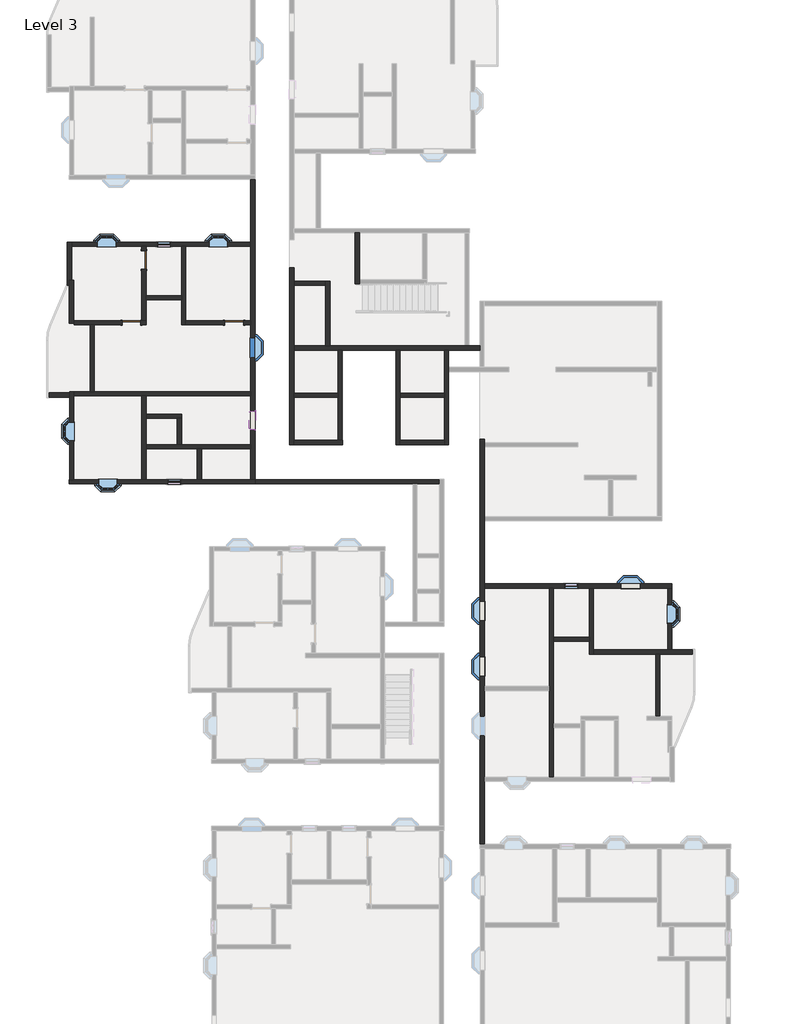
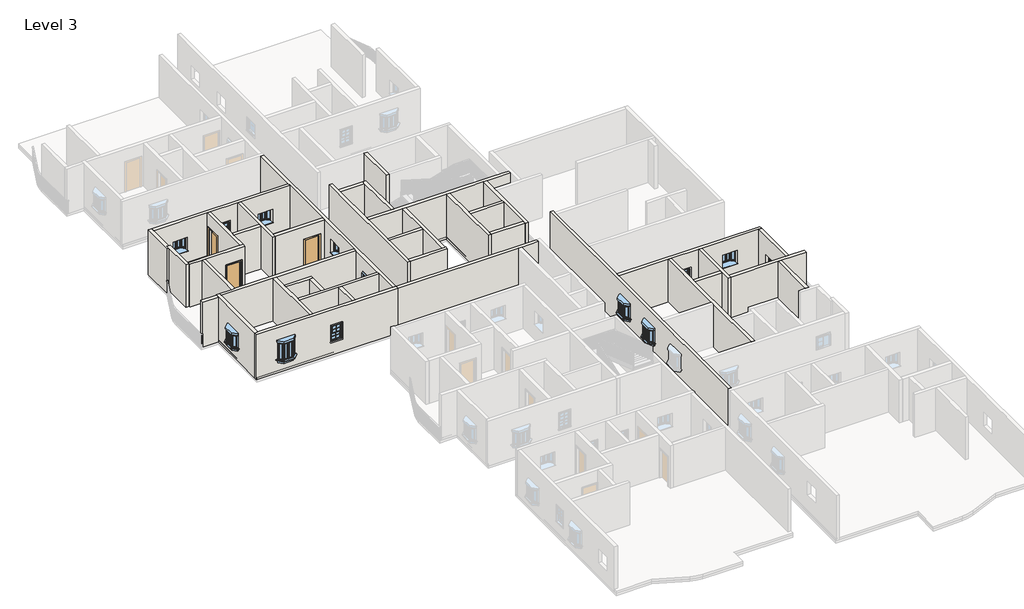
# One storey, part 3 of 14: 40 walls, 13 windows, 3 doors.
"""IFC4 building model written with IfcOpenShell, lengths in millimetres."""

from ifc_helpers import new_model, si_unit, frame, origin, place, context, project, spatial, polyline, outline, extrude, faceted_brep, transform, mapped, element, save
from components import door_54dd4da4, window_910x1210mm_154f9356, window_910x910mm_67ef725a, window_8debb0fa, windows_sgl_w_glazing_bars_910x910mm_256712d0

model = new_model("IFC4")

# Units and contexts
model_context = context("Model", 3, world=origin())
ifc_project = project(units=[si_unit("LENGTHUNIT", "METRE", prefix="MILLI")], contexts=[model_context])

# Site, building, storey
site = spatial("IfcSite", under=ifc_project)
building = spatial("IfcBuilding", under=site)
storey = spatial("IfcBuildingStorey", under=building, Name="Level 3", Elevation=6096.0)

# Doors
placement = place(None, origin())
door_shape = door_54dd4da4(model_context)
element("IfcDoor", 1, ObjectType="Single-Flush : 36\" x 84\"", at=placement, inside=storey, context=model_context, shape_type="MappedRepresentation", body=[
    mapped(door_shape, transform((-11210.3891351, 10605.7083494, 6096.0), x_axis=(1.0, 0.0, 0.0), y_axis=(0.0, 1.0, 0.0), z_axis=(0.0, 0.0, 1.0))),
])
element("IfcDoor", 2, ObjectType="Single-Flush : 36\" x 84\"", at=placement, inside=storey, context=model_context, shape_type="MappedRepresentation", body=[
    mapped(door_shape, transform((-15610.9391351, 13672.7583494, 6096.0), x_axis=(0.0, -1.0, 0.0), y_axis=(1.0, 0.0, 0.0), z_axis=(0.0, 0.0, 1.0))),
])
element("IfcDoor", 3, ObjectType="Single-Flush : 36\" x 84\"", at=placement, inside=storey, context=model_context, shape_type="MappedRepresentation", body=[
    mapped(door_shape, transform((-16220.5391351, 10605.7083494, 6096.0), x_axis=(1.0, 0.0, 0.0), y_axis=(0.0, 1.0, 0.0), z_axis=(0.0, 0.0, 1.0))),
])

# Walls
element("IfcWall", 4, ObjectType="4.5\" p", at=placement, inside=storey, context=model_context, shape_type="Brep", body=[
    faceted_brep([(-15509.3391351, 4456.3873146, 6096.0), (-13007.4391351, 4456.3873146, 6096.0), (-12804.2391351, 4456.3873146, 6096.0), (-10397.5891351, 4456.3873146, 6096.0), (-10397.5891351, 4456.3873146, 9144.0), (-12804.2391351, 4456.3873146, 9144.0), (-13007.4391351, 4456.3873146, 9144.0), (-15509.3391351, 4456.3873146, 9144.0), (-15509.3391351, 4659.5873146, 6096.0), (-15509.3391351, 4659.5873146, 9144.0), (-13985.3391351, 4659.5873146, 9144.0), (-13782.1391351, 4659.5873146, 9144.0), (-10397.5891351, 4659.5873146, 9144.0), (-10397.5891351, 4659.5873146, 6096.0), (-13782.1391351, 4659.5873146, 6096.0), (-13985.3391351, 4659.5873146, 6096.0)], [[[0, 1, 2, 3, 4, 5, 6, 7]], [[8, 9, 10, 11, 12, 13, 14, 15]], [[3, 2, 1, 0, 8, 15, 14, 13]], [[7, 6, 5, 4, 12, 11, 10, 9]], [[4, 3, 13, 12]], [[0, 7, 9, 8]]]),
])
element("IfcWall", 5, ObjectType="4.5\" p", at=placement, inside=storey, context=model_context, shape_type="SweptSolid", body=[
    extrude(outline(polyline([(-13007.4391351, 2953.9583494), (-13007.4391351, 4456.3873146), (-12804.2391351, 4456.3873146), (-12804.2391351, 2953.9583494), (-13007.4391351, 2953.9583494)])), frame((0.0, 0.0, 6096.0), z_axis=(0.0, 0.0, 1.0), x_axis=(1.0, 0.0, 0.0)), (0.0, 0.0, 1.0), 3048.0),
])
element("IfcWall", 6, ObjectType="4.5\" p", at=placement, inside=storey, context=model_context, shape_type="Brep", body=[
    faceted_brep([(-15509.3391351, 5953.2975261, 6096.0), (-13985.3391351, 5953.2975261, 6096.0), (-13782.1391351, 5953.2975261, 6096.0), (-13782.1391351, 5953.2975261, 9144.0), (-13985.3391351, 5953.2975261, 9144.0), (-15509.3391351, 5953.2975261, 9144.0), (-15509.3391351, 6156.4975261, 6096.0), (-15509.3391351, 6156.4975261, 9144.0), (-13782.1391351, 6156.4975261, 9144.0), (-13782.1391351, 6156.4975261, 6096.0)], [[[0, 1, 2, 3, 4, 5]], [[6, 7, 8, 9]], [[2, 1, 0, 6, 9]], [[5, 4, 3, 8, 7]], [[0, 5, 7, 6]], [[3, 2, 9, 8]]]),
])
element("IfcWall", 7, ObjectType="4.5\" p", at=placement, inside=storey, context=model_context, shape_type="SweptSolid", body=[
    extrude(outline(polyline([(-13985.3391351, 4659.5873146), (-13985.3391351, 5953.2975261), (-13782.1391351, 5953.2975261), (-13782.1391351, 4659.5873146), (-13985.3391351, 4659.5873146)])), frame((0.0, 0.0, 6096.0), z_axis=(0.0, 0.0, 1.0), x_axis=(1.0, 0.0, 0.0)), (0.0, 0.0, 1.0), 3048.0),
])
element("IfcWall", 8, ObjectType="4.5\" p", at=placement, inside=storey, context=model_context, shape_type="Brep", body=[
    faceted_brep([(-15712.5391351, 13215.5583494, 8229.6), (-15712.5391351, 13215.5583494, 6096.0), (-15712.5391351, 10707.3083494, 6096.0), (-15712.5391351, 10707.3083494, 9144.0), (-15712.5391351, 14333.1583494, 9144.0), (-15712.5391351, 14333.1583494, 6096.0), (-15712.5391351, 14129.9583494, 6096.0), (-15712.5391351, 14129.9583494, 8229.6), (-15509.3391351, 10707.3083494, 6096.0), (-15509.3391351, 11723.3083494, 6096.0), (-15509.3391351, 11926.5083494, 6096.0), (-15509.3391351, 13215.5583494, 6096.0), (-15509.3391351, 13215.5583494, 8229.6), (-15509.3391351, 14129.9583494, 8229.6), (-15509.3391351, 14129.9583494, 6096.0), (-15509.3391351, 14333.1583494, 6096.0), (-15509.3391351, 14333.1583494, 9144.0), (-15509.3391351, 11926.5083494, 9144.0), (-15509.3391351, 11723.3083494, 9144.0), (-15509.3391351, 10707.3083494, 9144.0)], [[[0, 1, 2, 3, 4, 5, 6, 7]], [[8, 9, 10, 11, 12, 13, 14, 15, 16, 17, 18, 19]], [[6, 5, 15, 14]], [[2, 1, 11, 10, 9, 8]], [[4, 3, 19, 18, 17, 16]], [[3, 2, 8, 19]], [[5, 4, 16, 15]], [[12, 11, 1, 0]], [[13, 12, 0, 7]], [[14, 13, 7, 6]]]),
])
element("IfcWall", 9, ObjectType="4.5\" p", at=placement, inside=storey, context=model_context, shape_type="Brep", body=[
    faceted_brep([(-13769.4391351, 14333.1583494, 6096.0), (-13769.4391351, 11926.5083494, 6096.0), (-13769.4391351, 11723.3083494, 6096.0), (-13769.4391351, 10504.1083494, 6096.0), (-13769.4391351, 10504.1083494, 9144.0), (-13769.4391351, 11723.3083494, 9144.0), (-13769.4391351, 11926.5083494, 9144.0), (-13769.4391351, 14333.1583494, 9144.0), (-13566.2391351, 14333.1583494, 6096.0), (-13566.2391351, 14333.1583494, 9144.0), (-13566.2391351, 10707.3083494, 9144.0), (-13566.2391351, 10504.1083494, 9144.0), (-13566.2391351, 10504.1083494, 6096.0), (-13566.2391351, 10707.3083494, 6096.0)], [[[0, 1, 2, 3, 4, 5, 6, 7]], [[8, 9, 10, 11, 12, 13]], [[3, 2, 1, 0, 8, 13, 12]], [[7, 6, 5, 4, 11, 10, 9]], [[0, 7, 9, 8]], [[4, 3, 12, 11]]]),
])
element("IfcWall", 10, ObjectType="4.5\" p", at=placement, inside=storey, context=model_context, shape_type="SweptSolid", body=[
    extrude(outline(polyline([(8229.6, -10753.1891351), (6096.0, -10753.1891351), (6096.0, -10397.5891351), (9144.0, -10397.5891351), (9144.0, -13566.2391351), (6096.0, -13566.2391351), (6096.0, -11667.5891351), (8229.6, -11667.5891351), (8229.6, -10753.1891351)])), frame((0.0, 10504.1083494, 0.0), z_axis=(0.0, 1.0, 0.0), x_axis=(0.0, 0.0, 1.0)), (0.0, 0.0, 1.0), 203.2),
])
element("IfcWall", 11, ObjectType="4.5\" p", at=placement, inside=storey, context=model_context, shape_type="SweptSolid", body=[
    extrude(outline(polyline([(-13769.4391351, 11723.3083494), (-15509.3391351, 11723.3083494), (-15509.3391351, 11926.5083494), (-13769.4391351, 11926.5083494), (-13769.4391351, 11723.3083494)])), frame((0.0, 0.0, 6096.0), z_axis=(0.0, 0.0, 1.0), x_axis=(1.0, 0.0, 0.0)), (0.0, 0.0, 1.0), 3048.0),
])
element("IfcWall", 12, ObjectType="4.5\" p", at=placement, inside=storey, context=model_context, shape_type="SweptSolid", body=[
    extrude(outline(polyline([(-6739.9891351, 12429.8715905), (-8289.3891351, 12429.8715905), (-8289.3891351, 12633.0715905), (-6739.9891351, 12633.0715905), (-6739.9891351, 12429.8715905)])), frame((0.0, 0.0, 6096.0), z_axis=(0.0, 0.0, 1.0), x_axis=(1.0, 0.0, 0.0)), (0.0, 0.0, 1.0), 3048.0),
])
element("IfcWall", 13, ObjectType="4.5\" p", at=placement, inside=storey, context=model_context, shape_type="SweptSolid", body=[
    extrude(outline(polyline([(-6130.3891351, 6970.2449943), (-8289.3891351, 6970.2449943), (-8289.3891351, 7173.4449943), (-6130.3891351, 7173.4449943), (-6130.3891351, 6970.2449943)])), frame((0.0, 0.0, 6096.0), z_axis=(0.0, 0.0, 1.0), x_axis=(1.0, 0.0, 0.0)), (0.0, 0.0, 1.0), 3048.0),
])
element("IfcWall", 14, ObjectType="4.5\" p", at=placement, inside=storey, context=model_context, shape_type="SweptSolid", body=[
    extrude(outline(polyline([(-948.7891351, 6970.2449943), (-3107.7891351, 6970.2449943), (-3107.7891351, 7173.4449943), (-948.7891351, 7173.4449943), (-948.7891351, 6970.2449943)])), frame((0.0, 0.0, 6096.0), z_axis=(0.0, 0.0, 1.0), x_axis=(1.0, 0.0, 0.0)), (0.0, 0.0, 1.0), 3048.0),
])
element("IfcWall", 15, ObjectType="4.5\" p", at=placement, inside=storey, context=model_context, shape_type="Brep", body=[
    faceted_brep([(-5298.5391351, 14988.9215905, 6096.0), (-5298.5391351, 12506.0715905, 6096.0), (-5298.5391351, 12506.0715905, 9144.0), (-5298.5391351, 14988.9215905, 9144.0), (-5095.3391351, 14988.9215905, 6096.0), (-5095.3391351, 14988.9215905, 9144.0), (-5095.3391351, 12709.2715905, 9144.0), (-5095.3391351, 12506.0715905, 9144.0), (-5095.3391351, 12506.0715905, 6096.0), (-5095.3391351, 12709.2715905, 6096.0)], [[[0, 1, 2, 3]], [[4, 5, 6, 7, 8, 9]], [[1, 0, 4, 9, 8]], [[3, 2, 7, 6, 5]], [[0, 3, 5, 4]], [[2, 1, 8, 7]]]),
])
element("IfcWall", 16, ObjectType="4.5\" p", at=placement, inside=storey, context=model_context, shape_type="SweptSolid", body=[
    extrude(outline(polyline([(-948.7891351, 4665.1949943), (-3107.7891351, 4665.1949943), (-3107.7891351, 4868.3949943), (-948.7891351, 4868.3949943), (-948.7891351, 4665.1949943)])), frame((0.0, 0.0, 6096.0), z_axis=(0.0, 0.0, 1.0), x_axis=(1.0, 0.0, 0.0)), (0.0, 0.0, 1.0), 3048.0),
])
element("IfcWall", 17, ObjectType="4.5\" p", at=placement, inside=storey, context=model_context, shape_type="Brep", body=[
    faceted_brep([(4184.4880523, -2336.4042694, 6096.0), (4184.4880523, -7130.6542694, 6096.0), (4184.4880523, -7333.8542694, 6096.0), (4184.4880523, -11556.6042694, 6096.0), (4184.4880523, -11556.6042694, 9144.0), (4184.4880523, -7333.8542694, 9144.0), (4184.4880523, -7130.6542694, 9144.0), (4184.4880523, -2336.4042694, 9144.0), (4387.6880523, -2336.4042694, 6096.0), (4387.6880523, -2336.4042694, 9144.0), (4387.6880523, -4736.7042694, 9144.0), (4387.6880523, -4939.9042694, 9144.0), (4387.6880523, -8959.4542694, 9144.0), (4387.6880523, -9162.6542694, 9144.0), (4387.6880523, -11556.6042694, 9144.0), (4387.6880523, -11556.6042694, 6096.0), (4387.6880523, -9162.6542694, 6096.0), (4387.6880523, -8959.4542694, 6096.0), (4387.6880523, -4939.9042694, 6096.0), (4387.6880523, -4736.7042694, 6096.0)], [[[0, 1, 2, 3, 4, 5, 6, 7]], [[8, 9, 10, 11, 12, 13, 14, 15, 16, 17, 18, 19]], [[3, 2, 1, 0, 8, 19, 18, 17, 16, 15]], [[7, 6, 5, 4, 14, 13, 12, 11, 10, 9]], [[4, 3, 15, 14]], [[0, 7, 9, 8]]]),
])
element("IfcWall", 18, ObjectType="4.5\" p", at=placement, inside=storey, context=model_context, shape_type="Brep", body=[
    faceted_brep([(803.8108649, 4915.2957306, 6096.0), (803.8108649, -14845.9042694, 6096.0), (803.8108649, -14845.9042694, 9144.0), (803.8108649, 4915.2957306, 9144.0), (803.8108649, -9516.0542694, 8206.0), (803.8108649, -9516.0542694, 7296.0), (803.8108649, -8606.0542694, 7296.0), (803.8108649, -8606.0542694, 8206.0), (803.8108649, -3909.0042694, 8206.0), (803.8108649, -3909.0042694, 7296.0), (803.8108649, -2999.0042694, 7296.0), (803.8108649, -2999.0042694, 8206.0), (803.8108649, -6620.4542694, 8206.0), (803.8108649, -6620.4542694, 7296.0), (803.8108649, -5710.4542694, 7296.0), (803.8108649, -5710.4542694, 8206.0), (1007.0108649, 4915.2957306, 6096.0), (1007.0108649, 4915.2957306, 9144.0), (1007.0108649, 4754.0949943, 9144.0), (1007.0108649, 4550.8949943, 9144.0), (1007.0108649, 1143.3957306, 9144.0), (1007.0108649, 940.1957306, 9144.0), (1007.0108649, -2133.2042694, 9144.0), (1007.0108649, -2336.4042694, 9144.0), (1007.0108649, -7130.6542694, 9144.0), (1007.0108649, -7333.8542694, 9144.0), (1007.0108649, -11556.6042694, 9144.0), (1007.0108649, -11759.8042694, 9144.0), (1007.0108649, -14845.9042694, 9144.0), (1007.0108649, -14845.9042694, 6096.0), (1007.0108649, -11759.8042694, 6096.0), (1007.0108649, -11556.6042694, 6096.0), (1007.0108649, -7333.8542694, 6096.0), (1007.0108649, -7130.6542694, 6096.0), (1007.0108649, -2336.4042694, 6096.0), (1007.0108649, -2133.2042694, 6096.0), (1007.0108649, 940.1957306, 6096.0), (1007.0108649, 1143.3957306, 6096.0), (1007.0108649, 4550.8949943, 6096.0), (1007.0108649, 4754.0949943, 6096.0), (1007.0108649, -9516.0542694, 8206.0), (1007.0108649, -8606.0542694, 8206.0), (1007.0108649, -8606.0542694, 7296.0), (1007.0108649, -9516.0542694, 7296.0), (1007.0108649, -3909.0042694, 8206.0), (1007.0108649, -2999.0042694, 8206.0), (1007.0108649, -2999.0042694, 7296.0), (1007.0108649, -3909.0042694, 7296.0), (1007.0108649, -6620.4542694, 8206.0), (1007.0108649, -5710.4542694, 8206.0), (1007.0108649, -5710.4542694, 7296.0), (1007.0108649, -6620.4542694, 7296.0)], [[[0, 1, 2, 3], [4, 5, 6, 7], [8, 9, 10, 11], [12, 13, 14, 15]], [[16, 17, 18, 19, 20, 21, 22, 23, 24, 25, 26, 27, 28, 29, 30, 31, 32, 33, 34, 35, 36, 37, 38, 39], [40, 41, 42, 43], [44, 45, 46, 47], [48, 49, 50, 51]], [[1, 0, 16, 39, 38, 37, 36, 35, 34, 33, 32, 31, 30, 29]], [[3, 2, 28, 27, 26, 25, 24, 23, 22, 21, 20, 19, 18, 17]], [[0, 3, 17, 16]], [[2, 1, 29, 28]], [[5, 4, 40, 43]], [[6, 5, 43, 42]], [[7, 6, 42, 41]], [[4, 7, 41, 40]], [[9, 8, 44, 47]], [[10, 9, 47, 46]], [[11, 10, 46, 45]], [[8, 11, 45, 44]], [[13, 12, 48, 51]], [[14, 13, 51, 50]], [[15, 14, 50, 49]], [[12, 15, 49, 48]]]),
])
element("IfcWall", 19, ObjectType="4.5\" p", at=placement, inside=storey, context=model_context, shape_type="SweptSolid", body=[
    extrude(outline(polyline([(6127.5880523, -4939.9042694), (4387.6880523, -4939.9042694), (4387.6880523, -4736.7042694), (6127.5880523, -4736.7042694), (6127.5880523, -4939.9042694)])), frame((0.0, 0.0, 6096.0), z_axis=(0.0, 0.0, 1.0), x_axis=(1.0, 0.0, 0.0)), (0.0, 0.0, 1.0), 3048.0),
])
element("IfcWall", 20, ObjectType="4.5\" p", at=placement, inside=storey, context=model_context, shape_type="Brep", body=[
    faceted_brep([(6127.5880523, -2336.4042694, 6096.0), (6127.5880523, -4736.7042694, 6096.0), (6127.5880523, -4939.9042694, 6096.0), (6127.5880523, -5555.8542694, 6096.0), (6127.5880523, -5555.8542694, 9144.0), (6127.5880523, -4939.9042694, 9144.0), (6127.5880523, -4736.7042694, 9144.0), (6127.5880523, -2336.4042694, 9144.0), (6330.7880523, -2336.4042694, 6096.0), (6330.7880523, -2336.4042694, 9144.0), (6330.7880523, -5352.6542694, 9144.0), (6330.7880523, -5555.8542694, 9144.0), (6330.7880523, -5555.8542694, 6096.0), (6330.7880523, -5352.6542694, 6096.0)], [[[0, 1, 2, 3, 4, 5, 6, 7]], [[8, 9, 10, 11, 12, 13]], [[3, 2, 1, 0, 8, 13, 12]], [[7, 6, 5, 4, 11, 10, 9]], [[0, 7, 9, 8]], [[4, 3, 12, 11]]]),
])
element("IfcWall", 21, ObjectType="4.5\" p", at=placement, inside=storey, context=model_context, shape_type="Brep", body=[
    faceted_brep([(6330.7880523, -5555.8542694, 6096.0), (9371.2322031, -5555.8542694, 6096.0), (9574.4322031, -5555.8542694, 6096.0), (11163.1380523, -5555.8542694, 6096.0), (11163.1380523, -5555.8542694, 9144.0), (9574.4322031, -5555.8542694, 9144.0), (9371.2322031, -5555.8542694, 9144.0), (6330.7880523, -5555.8542694, 9144.0), (6330.7880523, -5352.6542694, 6096.0), (6330.7880523, -5352.6542694, 9144.0), (9956.6380523, -5352.6542694, 9144.0), (10159.8380523, -5352.6542694, 9144.0), (11163.1380523, -5352.6542694, 9144.0), (11163.1380523, -5352.6542694, 6096.0), (10159.8380523, -5352.6542694, 6096.0), (9956.6380523, -5352.6542694, 6096.0)], [[[0, 1, 2, 3, 4, 5, 6, 7]], [[8, 9, 10, 11, 12, 13, 14, 15]], [[3, 2, 1, 0, 8, 15, 14, 13]], [[4, 3, 13, 12]], [[7, 6, 5, 4, 12, 11, 10, 9]], [[0, 7, 9, 8]]]),
])
element("IfcWall", 22, ObjectType="4.5\" p", at=placement, inside=storey, context=model_context, shape_type="SweptSolid", body=[
    extrude(outline(polyline([(9371.2322031, -8578.4542694), (9371.2322031, -5555.8542694), (9574.4322031, -5555.8542694), (9574.4322031, -8578.4542694), (9371.2322031, -8578.4542694)])), frame((0.0, 0.0, 6096.0), z_axis=(0.0, 0.0, 1.0), x_axis=(1.0, 0.0, 0.0)), (0.0, 0.0, 1.0), 3048.0),
])
element("IfcWall", 23, ObjectType="9\"", at=placement, inside=storey, context=model_context, shape_type="Brep", body=[
    faceted_brep([(-10181.6891351, 2953.9583494, 6096.0), (-10194.3891351, 2953.9583494, 6096.0), (-10397.5891351, 2953.9583494, 6096.0), (-12804.2391351, 2953.9583494, 6096.0), (-13007.4391351, 2953.9583494, 6096.0), (-15509.3391351, 2953.9583494, 6096.0), (-15712.5391351, 2953.9583494, 6096.0), (-19033.5891351, 2953.9583494, 6096.0), (-19236.7891351, 2953.9583494, 6096.0), (-19249.4891351, 2953.9583494, 6096.0), (-19249.4891351, 2953.9583494, 9144.0), (-19236.7891351, 2953.9583494, 9144.0), (-19033.5891351, 2953.9583494, 9144.0), (-15712.5391351, 2953.9583494, 9144.0), (-15509.3391351, 2953.9583494, 9144.0), (-13007.4391351, 2953.9583494, 9144.0), (-12804.2391351, 2953.9583494, 9144.0), (-10397.5891351, 2953.9583494, 9144.0), (-10194.3891351, 2953.9583494, 9144.0), (-10181.6891351, 2953.9583494, 9144.0), (-13794.8391351, 2953.9583494, 8077.2), (-14455.2391351, 2953.9583494, 8077.2), (-14455.2391351, 2953.9583494, 7010.4), (-13794.8391351, 2953.9583494, 7010.4), (-16918.0641351, 2953.9583494, 8220.4), (-17828.0641351, 2953.9583494, 8220.4), (-17828.0641351, 2953.9583494, 7010.4), (-16918.0641351, 2953.9583494, 7010.4), (-10181.6891351, 2750.7583494, 6096.0), (-10181.6891351, 2750.7583494, 9144.0), (-19249.4891351, 2750.7583494, 9144.0), (-19249.4891351, 2750.7583494, 6096.0), (-13794.8391351, 2750.7583494, 8077.2), (-13794.8391351, 2750.7583494, 7010.4), (-14455.2391351, 2750.7583494, 7010.4), (-14455.2391351, 2750.7583494, 8077.2), (-16918.0641351, 2750.7583494, 8220.4), (-16918.0641351, 2750.7583494, 7010.4), (-17828.0641351, 2750.7583494, 7010.4), (-17828.0641351, 2750.7583494, 8220.4)], [[[0, 1, 2, 3, 4, 5, 6, 7, 8, 9, 10, 11, 12, 13, 14, 15, 16, 17, 18, 19], [20, 21, 22, 23], [24, 25, 26, 27]], [[28, 29, 30, 31], [32, 33, 34, 35], [36, 37, 38, 39]], [[9, 8, 7, 6, 5, 4, 3, 2, 1, 0, 28, 31]], [[10, 9, 31, 30]], [[19, 18, 17, 16, 15, 14, 13, 12, 11, 10, 30, 29]], [[0, 19, 29, 28]], [[33, 32, 20, 23]], [[34, 33, 23, 22]], [[35, 34, 22, 21]], [[32, 35, 21, 20]], [[37, 36, 24, 27]], [[38, 37, 27, 26]], [[39, 38, 26, 25]], [[36, 39, 25, 24]]]),
])
element("IfcWall", 24, ObjectType="9\"", at=placement, inside=storey, context=model_context, shape_type="Brep", body=[
    faceted_brep([(-19033.5891351, 2953.9583494, 6096.0), (-19033.5891351, 7037.0083494, 6096.0), (-19033.5891351, 7240.2083494, 6096.0), (-19033.5891351, 7240.2083494, 9144.0), (-19033.5891351, 7037.0083494, 9144.0), (-19033.5891351, 2953.9583494, 9144.0), (-19033.5891351, 4854.8083494, 7920.4), (-19033.5891351, 5764.8083494, 7920.4), (-19033.5891351, 5764.8083494, 7010.4), (-19033.5891351, 4854.8083494, 7010.4), (-19236.7891351, 2953.9583494, 6096.0), (-19236.7891351, 2953.9583494, 9144.0), (-19236.7891351, 7240.2083494, 9144.0), (-19236.7891351, 7240.2083494, 6096.0), (-19236.7891351, 4854.8083494, 7920.4), (-19236.7891351, 4854.8083494, 7010.4), (-19236.7891351, 5764.8083494, 7010.4), (-19236.7891351, 5764.8083494, 7920.4)], [[[0, 1, 2, 3, 4, 5], [6, 7, 8, 9]], [[10, 11, 12, 13], [14, 15, 16, 17]], [[2, 1, 0, 10, 13]], [[5, 4, 3, 12, 11]], [[0, 5, 11, 10]], [[3, 2, 13, 12]], [[15, 14, 6, 9]], [[16, 15, 9, 8]], [[17, 16, 8, 7]], [[14, 17, 7, 6]]]),
])
element("IfcWall", 25, ObjectType="9\"", at=placement, inside=storey, context=model_context, shape_type="Brep", body=[
    faceted_brep([(-10194.3891351, 2953.9583494, 6096.0), (-10194.3891351, 17597.0583494, 6096.0), (-10194.3891351, 17597.0583494, 9144.0), (-10194.3891351, 2953.9583494, 9144.0), (-10194.3891351, 9841.5083494, 8206.0), (-10194.3891351, 9841.5083494, 7296.0), (-10194.3891351, 8931.5083494, 7296.0), (-10194.3891351, 8931.5083494, 8206.0), (-10194.3891351, 5393.297832, 8206.0), (-10194.3891351, 6303.297832, 8206.0), (-10194.3891351, 6303.297832, 7296.0), (-10194.3891351, 5393.297832, 7296.0), (-10397.5891351, 2953.9583494, 6096.0), (-10397.5891351, 2953.9583494, 9144.0), (-10397.5891351, 4456.3873146, 9144.0), (-10397.5891351, 4659.5873146, 9144.0), (-10397.5891351, 7037.0083494, 9144.0), (-10397.5891351, 7240.2083494, 9144.0), (-10397.5891351, 10504.1083494, 9144.0), (-10397.5891351, 10707.3083494, 9144.0), (-10397.5891351, 14333.1583494, 9144.0), (-10397.5891351, 14536.3583494, 9144.0), (-10397.5891351, 17597.0583494, 9144.0), (-10397.5891351, 17597.0583494, 6096.0), (-10397.5891351, 14536.3583494, 6096.0), (-10397.5891351, 14333.1583494, 6096.0), (-10397.5891351, 10707.3083494, 6096.0), (-10397.5891351, 10504.1083494, 6096.0), (-10397.5891351, 7240.2083494, 6096.0), (-10397.5891351, 7037.0083494, 6096.0), (-10397.5891351, 4659.5873146, 6096.0), (-10397.5891351, 4456.3873146, 6096.0), (-10397.5891351, 9841.5083494, 8206.0), (-10397.5891351, 8931.5083494, 8206.0), (-10397.5891351, 8931.5083494, 7296.0), (-10397.5891351, 9841.5083494, 7296.0), (-10397.5891351, 5393.297832, 8206.0), (-10397.5891351, 5393.297832, 7296.0), (-10397.5891351, 6303.297832, 7296.0), (-10397.5891351, 6303.297832, 8206.0)], [[[0, 1, 2, 3], [4, 5, 6, 7], [8, 9, 10, 11]], [[12, 13, 14, 15, 16, 17, 18, 19, 20, 21, 22, 23, 24, 25, 26, 27, 28, 29, 30, 31], [32, 33, 34, 35], [36, 37, 38, 39]], [[1, 0, 12, 31, 30, 29, 28, 27, 26, 25, 24, 23]], [[2, 1, 23, 22]], [[3, 2, 22, 21, 20, 19, 18, 17, 16, 15, 14, 13]], [[0, 3, 13, 12]], [[5, 4, 32, 35]], [[6, 5, 35, 34]], [[7, 6, 34, 33]], [[4, 7, 33, 32]], [[37, 36, 8, 11]], [[38, 37, 11, 10]], [[39, 38, 10, 9]], [[36, 39, 9, 8]]]),
])
element("IfcWall", 26, ObjectType="9\"", at=placement, inside=storey, context=model_context, shape_type="SweptSolid", body=[
    extrude(outline(polyline([(-19249.4891351, 6979.8583494), (-20240.0891351, 6979.8583494), (-20240.0891351, 7183.0583494), (-19249.4891351, 7183.0583494), (-19249.4891351, 6979.8583494)])), frame((0.0, 0.0, 6096.0), z_axis=(0.0, 0.0, 1.0), x_axis=(1.0, 0.0, 0.0)), (0.0, 0.0, 1.0), 3048.0),
])
element("IfcWall", 27, ObjectType="9\"", at=placement, inside=storey, context=model_context, shape_type="Brep", body=[
    faceted_brep([(-19147.8891351, 12435.1858981, 6096.0), (-19147.8891351, 14333.1583494, 6096.0), (-19147.8891351, 14536.3583494, 6096.0), (-19147.8891351, 14549.0583494, 6096.0), (-19147.8891351, 14549.0583494, 9144.0), (-19147.8891351, 14536.3583494, 9144.0), (-19147.8891351, 14333.1583494, 9144.0), (-19147.8891351, 12435.1858981, 9144.0), (-19351.0891351, 12435.1858981, 6096.0), (-19351.0891351, 12435.1858981, 9144.0), (-19351.0891351, 14549.0583494, 9144.0), (-19351.0891351, 14549.0583494, 6096.0)], [[[0, 1, 2, 3, 4, 5, 6, 7]], [[8, 9, 10, 11]], [[3, 2, 1, 0, 8, 11]], [[4, 3, 11, 10]], [[7, 6, 5, 4, 10, 9]], [[0, 7, 9, 8]]]),
])
element("IfcWall", 28, ObjectType="9\"", at=placement, inside=storey, context=model_context, shape_type="Brep", body=[
    faceted_brep([(-19147.8891351, 14333.1583494, 6096.0), (-15712.5391351, 14333.1583494, 6096.0), (-15509.3391351, 14333.1583494, 6096.0), (-13769.4391351, 14333.1583494, 6096.0), (-13566.2391351, 14333.1583494, 6096.0), (-10397.5891351, 14333.1583494, 6096.0), (-10397.5891351, 14333.1583494, 9144.0), (-13566.2391351, 14333.1583494, 9144.0), (-13769.4391351, 14333.1583494, 9144.0), (-15509.3391351, 14333.1583494, 9144.0), (-15712.5391351, 14333.1583494, 9144.0), (-19147.8891351, 14333.1583494, 9144.0), (-17885.2141351, 14333.1583494, 7920.4), (-16975.2141351, 14333.1583494, 7920.4), (-16975.2141351, 14333.1583494, 7010.4), (-17885.2141351, 14333.1583494, 7010.4), (-12436.9141351, 14333.1583494, 7920.4), (-11526.9141351, 14333.1583494, 7920.4), (-11526.9141351, 14333.1583494, 7010.4), (-12436.9141351, 14333.1583494, 7010.4), (-14309.1891351, 14333.1583494, 8077.2), (-14309.1891351, 14333.1583494, 7010.4), (-14969.5891351, 14333.1583494, 7010.4), (-14969.5891351, 14333.1583494, 8077.2), (-19147.8891351, 14536.3583494, 6096.0), (-19147.8891351, 14536.3583494, 9144.0), (-10397.5891351, 14536.3583494, 9144.0), (-10397.5891351, 14536.3583494, 6096.0), (-17885.2141351, 14536.3583494, 7920.4), (-17885.2141351, 14536.3583494, 7010.4), (-16975.2141351, 14536.3583494, 7010.4), (-16975.2141351, 14536.3583494, 7920.4), (-12436.9141351, 14536.3583494, 7920.4), (-12436.9141351, 14536.3583494, 7010.4), (-11526.9141351, 14536.3583494, 7010.4), (-11526.9141351, 14536.3583494, 7920.4), (-14309.1891351, 14536.3583494, 8077.2), (-14969.5891351, 14536.3583494, 8077.2), (-14969.5891351, 14536.3583494, 7010.4), (-14309.1891351, 14536.3583494, 7010.4)], [[[0, 1, 2, 3, 4, 5, 6, 7, 8, 9, 10, 11], [12, 13, 14, 15], [16, 17, 18, 19], [20, 21, 22, 23]], [[24, 25, 26, 27], [28, 29, 30, 31], [32, 33, 34, 35], [36, 37, 38, 39]], [[5, 4, 3, 2, 1, 0, 24, 27]], [[11, 10, 9, 8, 7, 6, 26, 25]], [[6, 5, 27, 26]], [[0, 11, 25, 24]], [[29, 28, 12, 15]], [[30, 29, 15, 14]], [[31, 30, 14, 13]], [[28, 31, 13, 12]], [[33, 32, 16, 19]], [[34, 33, 19, 18]], [[35, 34, 18, 17]], [[32, 35, 17, 16]], [[21, 20, 36, 39]], [[22, 21, 39, 38]], [[23, 22, 38, 37]], [[20, 23, 37, 36]]]),
])
element("IfcWall", 29, ObjectType="9\"", at=placement, inside=storey, context=model_context, shape_type="SweptSolid", body=[
    extrude(outline(polyline([(-19249.4891351, 10585.5474528), (-19249.4891351, 12672.4473407), (-19046.2891351, 12672.4473407), (-19046.2891351, 10585.5474528), (-19249.4891351, 10585.5474528)])), frame((0.0, 0.0, 6096.0), z_axis=(0.0, 0.0, 1.0), x_axis=(1.0, 0.0, 0.0)), (0.0, 0.0, 1.0), 3048.0),
])
element("IfcWall", 30, ObjectType="9\" w", at=placement, inside=storey, context=model_context, shape_type="Brep", body=[
    faceted_brep([(-1177.3891351, 2953.9583494, 6096.0), (-10181.6891351, 2953.9583494, 6096.0), (-10181.6891351, 2953.9583494, 9144.0), (-1177.3891351, 2953.9583494, 9144.0), (-1177.3891351, 2750.7583494, 6096.0), (-1177.3891351, 2750.7583494, 9144.0), (-2269.5891351, 2750.7583494, 9144.0), (-2472.7891351, 2750.7583494, 9144.0), (-10181.6891351, 2750.7583494, 9144.0), (-10181.6891351, 2750.7583494, 6096.0), (-2472.7891351, 2750.7583494, 6096.0), (-2269.5891351, 2750.7583494, 6096.0)], [[[0, 1, 2, 3]], [[4, 5, 6, 7, 8, 9, 10, 11]], [[1, 0, 4, 11, 10, 9]], [[2, 1, 9, 8]], [[3, 2, 8, 7, 6, 5]], [[0, 3, 5, 4]]]),
])
element("IfcWall", 31, ObjectType="9\" w", at=placement, inside=storey, context=model_context, shape_type="Brep", body=[
    faceted_brep([(-15763.3391351, 10504.1083494, 8229.6), (-15763.3391351, 10504.1083494, 6096.0), (-15509.3391351, 10504.1083494, 6096.0), (-15509.3391351, 10504.1083494, 9144.0), (-18042.9891351, 10504.1083494, 9144.0), (-18246.1891351, 10504.1083494, 9144.0), (-19027.2391351, 10504.1083494, 9144.0), (-19027.2391351, 10504.1083494, 6096.0), (-18246.1891351, 10504.1083494, 6096.0), (-18042.9891351, 10504.1083494, 6096.0), (-16677.7391351, 10504.1083494, 6096.0), (-16677.7391351, 10504.1083494, 8229.6), (-15509.3391351, 10707.3083494, 6096.0), (-15712.5391351, 10707.3083494, 6096.0), (-15763.3391351, 10707.3083494, 6096.0), (-15763.3391351, 10707.3083494, 8229.6), (-16677.7391351, 10707.3083494, 8229.6), (-16677.7391351, 10707.3083494, 6096.0), (-19027.2391351, 10707.3083494, 6096.0), (-19027.2391351, 10707.3083494, 9144.0), (-15712.5391351, 10707.3083494, 9144.0), (-15509.3391351, 10707.3083494, 9144.0)], [[[0, 1, 2, 3, 4, 5, 6, 7, 8, 9, 10, 11]], [[12, 13, 14, 15, 16, 17, 18, 19, 20, 21]], [[2, 1, 14, 13, 12]], [[10, 9, 8, 7, 18, 17]], [[6, 5, 4, 3, 21, 20, 19]], [[7, 6, 19, 18]], [[3, 2, 12, 21]], [[15, 14, 1, 0]], [[16, 15, 0, 11]], [[17, 16, 11, 10]]]),
])
element("IfcWall", 32, ObjectType="9\" w", at=placement, inside=storey, context=model_context, shape_type="SweptSolid", body=[
    extrude(outline(polyline([(-18246.1891351, 7240.2083494), (-18246.1891351, 10504.1083494), (-18042.9891351, 10504.1083494), (-18042.9891351, 7240.2083494), (-18246.1891351, 7240.2083494)])), frame((0.0, 0.0, 6096.0), z_axis=(0.0, 0.0, 1.0), x_axis=(1.0, 0.0, 0.0)), (0.0, 0.0, 1.0), 3048.0),
])
element("IfcWall", 33, ObjectType="9\" w", at=placement, inside=storey, context=model_context, shape_type="Brep", body=[
    faceted_brep([(-19033.5891351, 7037.0083494, 6096.0), (-15712.5391351, 7037.0083494, 6096.0), (-15509.3391351, 7037.0083494, 6096.0), (-10397.5891351, 7037.0083494, 6096.0), (-10397.5891351, 7037.0083494, 9144.0), (-15509.3391351, 7037.0083494, 9144.0), (-15712.5391351, 7037.0083494, 9144.0), (-19033.5891351, 7037.0083494, 9144.0), (-19033.5891351, 7240.2083494, 6096.0), (-19033.5891351, 7240.2083494, 9144.0), (-18246.1891351, 7240.2083494, 9144.0), (-18042.9891351, 7240.2083494, 9144.0), (-10397.5891351, 7240.2083494, 9144.0), (-10397.5891351, 7240.2083494, 6096.0), (-18042.9891351, 7240.2083494, 6096.0), (-18246.1891351, 7240.2083494, 6096.0)], [[[0, 1, 2, 3, 4, 5, 6, 7]], [[8, 9, 10, 11, 12, 13, 14, 15]], [[3, 2, 1, 0, 8, 15, 14, 13]], [[7, 6, 5, 4, 12, 11, 10, 9]], [[0, 7, 9, 8]], [[4, 3, 13, 12]]]),
])
element("IfcWall", 34, ObjectType="9\" w", at=placement, inside=storey, context=model_context, shape_type="Brep", body=[
    faceted_brep([(-15712.5391351, 7037.0083494, 6096.0), (-15712.5391351, 2953.9583494, 6096.0), (-15712.5391351, 2953.9583494, 9144.0), (-15712.5391351, 7037.0083494, 9144.0), (-15509.3391351, 7037.0083494, 6096.0), (-15509.3391351, 7037.0083494, 9144.0), (-15509.3391351, 6156.4975261, 9144.0), (-15509.3391351, 5953.2975261, 9144.0), (-15509.3391351, 4659.5873146, 9144.0), (-15509.3391351, 4456.3873146, 9144.0), (-15509.3391351, 2953.9583494, 9144.0), (-15509.3391351, 2953.9583494, 6096.0), (-15509.3391351, 4456.3873146, 6096.0), (-15509.3391351, 4659.5873146, 6096.0), (-15509.3391351, 5953.2975261, 6096.0), (-15509.3391351, 6156.4975261, 6096.0)], [[[0, 1, 2, 3]], [[4, 5, 6, 7, 8, 9, 10, 11, 12, 13, 14, 15]], [[1, 0, 4, 15, 14, 13, 12, 11]], [[3, 2, 10, 9, 8, 7, 6, 5]], [[2, 1, 11, 10]], [[0, 3, 5, 4]]]),
])
element("IfcWall", 35, ObjectType="9\" w", at=placement, inside=storey, context=model_context, shape_type="Brep", body=[
    faceted_brep([(-8492.5891351, 13295.1410318, 6096.0), (-8492.5891351, 4652.4949943, 6096.0), (-8492.5891351, 4652.4949943, 9144.0), (-8492.5891351, 13295.1410318, 9144.0), (-8289.3891351, 13295.1410318, 6096.0), (-8289.3891351, 13295.1410318, 9144.0), (-8289.3891351, 12633.0715905, 9144.0), (-8289.3891351, 12429.8715905, 9144.0), (-8289.3891351, 9478.4949943, 9144.0), (-8289.3891351, 9275.2949943, 9144.0), (-8289.3891351, 7173.4449943, 9144.0), (-8289.3891351, 6970.2449943, 9144.0), (-8289.3891351, 4868.3949943, 9144.0), (-8289.3891351, 4665.1949943, 9144.0), (-8289.3891351, 4652.4949943, 9144.0), (-8289.3891351, 4652.4949943, 6096.0), (-8289.3891351, 4665.1949943, 6096.0), (-8289.3891351, 4868.3949943, 6096.0), (-8289.3891351, 6970.2449943, 6096.0), (-8289.3891351, 7173.4449943, 6096.0), (-8289.3891351, 9275.2949943, 6096.0), (-8289.3891351, 9478.4949943, 6096.0), (-8289.3891351, 12429.8715905, 6096.0), (-8289.3891351, 12633.0715905, 6096.0)], [[[0, 1, 2, 3]], [[4, 5, 6, 7, 8, 9, 10, 11, 12, 13, 14, 15, 16, 17, 18, 19, 20, 21, 22, 23]], [[1, 0, 4, 23, 22, 21, 20, 19, 18, 17, 16, 15]], [[2, 1, 15, 14]], [[3, 2, 14, 13, 12, 11, 10, 9, 8, 7, 6, 5]], [[0, 3, 5, 4]]]),
])
element("IfcWall", 36, ObjectType="9\" w", at=placement, inside=storey, context=model_context, shape_type="Brep", body=[
    faceted_brep([(-8289.3891351, 4665.1949943, 6096.0), (-5914.4891351, 4665.1949943, 6096.0), (-5914.4891351, 4665.1949943, 9144.0), (-8289.3891351, 4665.1949943, 9144.0), (-8289.3891351, 4868.3949943, 6096.0), (-8289.3891351, 4868.3949943, 9144.0), (-6130.3891351, 4868.3949943, 9144.0), (-5927.1891351, 4868.3949943, 9144.0), (-5914.4891351, 4868.3949943, 9144.0), (-5914.4891351, 4868.3949943, 6096.0), (-5927.1891351, 4868.3949943, 6096.0), (-6130.3891351, 4868.3949943, 6096.0)], [[[0, 1, 2, 3]], [[4, 5, 6, 7, 8, 9, 10, 11]], [[1, 0, 4, 11, 10, 9]], [[2, 1, 9, 8]], [[3, 2, 8, 7, 6, 5]], [[0, 3, 5, 4]]]),
])
element("IfcWall", 37, ObjectType="9\" w", at=placement, inside=storey, context=model_context, shape_type="Brep", body=[
    faceted_brep([(-5927.1891351, 4868.3949943, 6096.0), (-5927.1891351, 9275.2949943, 6096.0), (-5927.1891351, 9275.2949943, 9144.0), (-5927.1891351, 4868.3949943, 9144.0), (-6130.3891351, 4868.3949943, 6096.0), (-6130.3891351, 4868.3949943, 9144.0), (-6130.3891351, 6970.2449943, 9144.0), (-6130.3891351, 7173.4449943, 9144.0), (-6130.3891351, 9275.2949943, 9144.0), (-6130.3891351, 9275.2949943, 6096.0), (-6130.3891351, 7173.4449943, 6096.0), (-6130.3891351, 6970.2449943, 6096.0)], [[[0, 1, 2, 3]], [[4, 5, 6, 7, 8, 9, 10, 11]], [[1, 0, 4, 11, 10, 9]], [[3, 2, 8, 7, 6, 5]], [[0, 3, 5, 4]], [[2, 1, 9, 8]]]),
])
element("IfcWall", 38, ObjectType="9\" w", at=placement, inside=storey, context=model_context, shape_type="Brep", body=[
    faceted_brep([(-8289.3891351, 9275.2949943, 6096.0), (-6130.3891351, 9275.2949943, 6096.0), (-5927.1891351, 9275.2949943, 6096.0), (-3310.9891351, 9275.2949943, 6096.0), (-3107.7891351, 9275.2949943, 6096.0), (-948.7891351, 9275.2949943, 6096.0), (-745.5891351, 9275.2949943, 6096.0), (793.5880523, 9275.2949943, 6096.0), (793.5880523, 9275.2949943, 9144.0), (-745.5891351, 9275.2949943, 9144.0), (-948.7891351, 9275.2949943, 9144.0), (-3107.7891351, 9275.2949943, 9144.0), (-3310.9891351, 9275.2949943, 9144.0), (-5927.1891351, 9275.2949943, 9144.0), (-6130.3891351, 9275.2949943, 9144.0), (-8289.3891351, 9275.2949943, 9144.0), (-8289.3891351, 9478.4949943, 6096.0), (-8289.3891351, 9478.4949943, 9144.0), (-6739.9891351, 9478.4949943, 9144.0), (-6536.7891351, 9478.4949943, 9144.0), (54.5108649, 9478.4949943, 9144.0), (257.7108649, 9478.4949943, 9144.0), (793.5880523, 9478.4949943, 9144.0), (793.5880523, 9478.4949943, 6096.0), (257.7108649, 9478.4949943, 6096.0), (54.5108649, 9478.4949943, 6096.0), (-6536.7891351, 9478.4949943, 6096.0), (-6739.9891351, 9478.4949943, 6096.0)], [[[0, 1, 2, 3, 4, 5, 6, 7, 8, 9, 10, 11, 12, 13, 14, 15]], [[16, 17, 18, 19, 20, 21, 22, 23, 24, 25, 26, 27]], [[7, 6, 5, 4, 3, 2, 1, 0, 16, 27, 26, 25, 24, 23]], [[15, 14, 13, 12, 11, 10, 9, 8, 22, 21, 20, 19, 18, 17]], [[0, 15, 17, 16]], [[8, 7, 23, 22]]]),
])
element("IfcWall", 39, ObjectType="9\" w", at=placement, inside=storey, context=model_context, shape_type="Brep", body=[
    faceted_brep([(-3310.9891351, 9275.2949943, 6096.0), (-3310.9891351, 4652.4949943, 6096.0), (-3310.9891351, 4652.4949943, 9144.0), (-3310.9891351, 9275.2949943, 9144.0), (-3107.7891351, 9275.2949943, 6096.0), (-3107.7891351, 9275.2949943, 9144.0), (-3107.7891351, 7173.4449943, 9144.0), (-3107.7891351, 6970.2449943, 9144.0), (-3107.7891351, 4868.3949943, 9144.0), (-3107.7891351, 4665.1949943, 9144.0), (-3107.7891351, 4652.4949943, 9144.0), (-3107.7891351, 4652.4949943, 6096.0), (-3107.7891351, 4665.1949943, 6096.0), (-3107.7891351, 4868.3949943, 6096.0), (-3107.7891351, 6970.2449943, 6096.0), (-3107.7891351, 7173.4449943, 6096.0)], [[[0, 1, 2, 3]], [[4, 5, 6, 7, 8, 9, 10, 11, 12, 13, 14, 15]], [[1, 0, 4, 15, 14, 13, 12, 11]], [[2, 1, 11, 10]], [[3, 2, 10, 9, 8, 7, 6, 5]], [[0, 3, 5, 4]]]),
])
element("IfcWall", 40, ObjectType="9\" w", at=placement, inside=storey, context=model_context, shape_type="Brep", body=[
    faceted_brep([(-745.5891351, 4652.4949943, 6096.0), (-745.5891351, 8223.6457306, 6096.0), (-745.5891351, 8426.8457306, 6096.0), (-745.5891351, 9275.2949943, 6096.0), (-745.5891351, 9275.2949943, 9144.0), (-745.5891351, 8426.8457306, 9144.0), (-745.5891351, 8223.6457306, 9144.0), (-745.5891351, 4652.4949943, 9144.0), (-948.7891351, 4652.4949943, 6096.0), (-948.7891351, 4652.4949943, 9144.0), (-948.7891351, 4665.1949943, 9144.0), (-948.7891351, 4868.3949943, 9144.0), (-948.7891351, 6970.2449943, 9144.0), (-948.7891351, 7173.4449943, 9144.0), (-948.7891351, 9275.2949943, 9144.0), (-948.7891351, 9275.2949943, 6096.0), (-948.7891351, 7173.4449943, 6096.0), (-948.7891351, 6970.2449943, 6096.0), (-948.7891351, 4868.3949943, 6096.0), (-948.7891351, 4665.1949943, 6096.0)], [[[0, 1, 2, 3, 4, 5, 6, 7]], [[8, 9, 10, 11, 12, 13, 14, 15, 16, 17, 18, 19]], [[3, 2, 1, 0, 8, 19, 18, 17, 16, 15]], [[7, 6, 5, 4, 14, 13, 12, 11, 10, 9]], [[0, 7, 9, 8]], [[4, 3, 15, 14]]]),
])
element("IfcWall", 41, ObjectType="9\" w", at=placement, inside=storey, context=model_context, shape_type="Brep", body=[
    faceted_brep([(-6536.7891351, 9478.4949943, 6096.0), (-6536.7891351, 12633.0715905, 6096.0), (-6536.7891351, 12633.0715905, 9144.0), (-6536.7891351, 9478.4949943, 9144.0), (-6739.9891351, 9478.4949943, 6096.0), (-6739.9891351, 9478.4949943, 9144.0), (-6739.9891351, 12429.8715905, 9144.0), (-6739.9891351, 12633.0715905, 9144.0), (-6739.9891351, 12633.0715905, 6096.0), (-6739.9891351, 12429.8715905, 6096.0)], [[[0, 1, 2, 3]], [[4, 5, 6, 7, 8, 9]], [[1, 0, 4, 9, 8]], [[3, 2, 7, 6, 5]], [[0, 3, 5, 4]], [[2, 1, 8, 7]]]),
])
element("IfcWall", 42, ObjectType="9\" w", at=placement, inside=storey, context=model_context, shape_type="Brep", body=[
    faceted_brep([(1007.0108649, -2336.4042694, 6096.0), (4184.4880523, -2336.4042694, 6096.0), (4387.6880523, -2336.4042694, 6096.0), (6127.5880523, -2336.4042694, 6096.0), (6330.7880523, -2336.4042694, 6096.0), (9956.6380523, -2336.4042694, 6096.0), (10159.8380523, -2336.4042694, 6096.0), (10172.5380523, -2336.4042694, 6096.0), (10172.5380523, -2336.4042694, 9144.0), (10159.8380523, -2336.4042694, 9144.0), (9956.6380523, -2336.4042694, 9144.0), (6330.7880523, -2336.4042694, 9144.0), (6127.5880523, -2336.4042694, 9144.0), (4387.6880523, -2336.4042694, 9144.0), (4184.4880523, -2336.4042694, 9144.0), (1007.0108649, -2336.4042694, 9144.0), (7688.7130523, -2336.4042694, 8206.0), (8598.7130523, -2336.4042694, 8206.0), (8598.7130523, -2336.4042694, 7296.0), (7688.7130523, -2336.4042694, 7296.0), (4927.4380523, -2336.4042694, 8077.2), (5587.8380523, -2336.4042694, 8077.2), (5587.8380523, -2336.4042694, 7010.4), (4927.4380523, -2336.4042694, 7010.4), (1007.0108649, -2133.2042694, 6096.0), (1007.0108649, -2133.2042694, 9144.0), (10172.5380523, -2133.2042694, 9144.0), (10172.5380523, -2133.2042694, 6096.0), (7688.7130523, -2133.2042694, 8206.0), (7688.7130523, -2133.2042694, 7296.0), (8598.7130523, -2133.2042694, 7296.0), (8598.7130523, -2133.2042694, 8206.0), (4927.4380523, -2133.2042694, 8077.2), (4927.4380523, -2133.2042694, 7010.4), (5587.8380523, -2133.2042694, 7010.4), (5587.8380523, -2133.2042694, 8077.2)], [[[0, 1, 2, 3, 4, 5, 6, 7, 8, 9, 10, 11, 12, 13, 14, 15], [16, 17, 18, 19], [20, 21, 22, 23]], [[24, 25, 26, 27], [28, 29, 30, 31], [32, 33, 34, 35]], [[7, 6, 5, 4, 3, 2, 1, 0, 24, 27]], [[8, 7, 27, 26]], [[15, 14, 13, 12, 11, 10, 9, 8, 26, 25]], [[0, 15, 25, 24]], [[29, 28, 16, 19]], [[30, 29, 19, 18]], [[31, 30, 18, 17]], [[28, 31, 17, 16]], [[33, 32, 20, 23]], [[34, 33, 23, 22]], [[35, 34, 22, 21]], [[32, 35, 21, 20]]]),
])
element("IfcWall", 43, ObjectType="9\" w", at=placement, inside=storey, context=model_context, shape_type="SweptSolid", body=[
    extrude(outline(polyline([(-2336.4042694, 6096.0), (-5352.6542694, 6096.0), (-5352.6542694, 9144.0), (-2336.4042694, 9144.0), (-2336.4042694, 6096.0)]), holes=[polyline([(-3151.4042694, 7920.4), (-4061.4042694, 7920.4), (-4061.4042694, 7010.4), (-3151.4042694, 7010.4), (-3151.4042694, 7920.4)])]), frame((9956.6380523, 0.0, 0.0), z_axis=(1.0, 0.0, 0.0), x_axis=(0.0, 1.0, 0.0)), (0.0, 0.0, 1.0), 203.2),
])

# Windows
window_910x1210mm_shape = window_910x1210mm_154f9356(model_context)
element("IfcWindow", 44, ObjectType="910x1210mm", at=placement, inside=storey, context=model_context, shape_type="MappedRepresentation", body=[
    mapped(window_910x1210mm_shape, transform((-17943.0641351, 2860.8149172, 6110.4), x_axis=(-1.0, 0.0, 0.0), y_axis=(0.0, -1.0, 0.0), z_axis=(0.0, 0.0, 1.0))),
])
window_910x910mm_shape = window_910x910mm_67ef725a(model_context)
element("IfcWindow", 45, ObjectType="910x910mm", at=placement, inside=storey, context=model_context, shape_type="MappedRepresentation", body=[
    mapped(window_910x910mm_shape, transform((8713.7130523, -2243.2608372, 6096.0), x_axis=(1.0, 0.0, 0.0), y_axis=(0.0, 1.0, 0.0), z_axis=(0.0, 0.0, 1.0))),
])
element("IfcWindow", 46, ObjectType="910x910mm", at=placement, inside=storey, context=model_context, shape_type="MappedRepresentation", body=[
    mapped(window_910x910mm_shape, transform((10049.7814845, -4176.4042694, 5810.4), x_axis=(0.0, -1.0, 0.0), y_axis=(1.0, 0.0, 0.0), z_axis=(0.0, 0.0, 1.0))),
])
element("IfcWindow", 47, ObjectType="910x910mm", at=placement, inside=storey, context=model_context, shape_type="MappedRepresentation", body=[
    mapped(window_910x910mm_shape, transform((-16860.2141351, 14426.3017816, 5810.4), x_axis=(1.0, 0.0, 0.0), y_axis=(0.0, 1.0, 0.0), z_axis=(0.0, 0.0, 1.0))),
])
element("IfcWindow", 48, ObjectType="910x910mm", at=placement, inside=storey, context=model_context, shape_type="MappedRepresentation", body=[
    mapped(window_910x910mm_shape, transform((-11411.9141351, 14426.3017816, 5810.4), x_axis=(1.0, 0.0, 0.0), y_axis=(0.0, 1.0, 0.0), z_axis=(0.0, 0.0, 1.0))),
])
element("IfcWindow", 49, ObjectType="910x910mm", at=placement, inside=storey, context=model_context, shape_type="MappedRepresentation", body=[
    mapped(window_910x910mm_shape, transform((-10304.445703, 8816.5083494, 6096.0), x_axis=(0.0, -1.0, 0.0), y_axis=(1.0, 0.0, 0.0), z_axis=(0.0, 0.0, 1.0))),
])
element("IfcWindow", 50, ObjectType="910x910mm", at=placement, inside=storey, context=model_context, shape_type="MappedRepresentation", body=[
    mapped(window_910x910mm_shape, transform((-19126.7325673, 5879.8083494, 5810.4), x_axis=(0.0, 1.0, 0.0), y_axis=(-1.0, 0.0, 0.0), z_axis=(0.0, 0.0, 1.0))),
])
element("IfcWindow", 51, ObjectType="910x910mm", at=placement, inside=storey, context=model_context, shape_type="MappedRepresentation", body=[
    mapped(window_910x910mm_shape, transform((913.8674327, -2884.0042694, 6096.0), x_axis=(0.0, 1.0, 0.0), y_axis=(-1.0, 0.0, 0.0), z_axis=(0.0, 0.0, 1.0))),
])
element("IfcWindow", 52, ObjectType="910x910mm", at=placement, inside=storey, context=model_context, shape_type="MappedRepresentation", body=[
    mapped(window_910x910mm_shape, transform((913.8674327, -5595.4542694, 6096.0), x_axis=(0.0, 1.0, 0.0), y_axis=(-1.0, 0.0, 0.0), z_axis=(0.0, 0.0, 1.0))),
])
window_shape = window_8debb0fa(model_context)
element("IfcWindow", 53, ObjectType="Window-Double-Hung : 26\" x 42\"", at=placement, inside=storey, context=model_context, shape_type="MappedRepresentation", body=[
    mapped(window_shape, transform((5257.6380523, -2234.8042694, 6096.0), x_axis=(1.0, 0.0, 0.0), y_axis=(0.0, 1.0, 0.0), z_axis=(0.0, 0.0, 1.0))),
])
element("IfcWindow", 54, ObjectType="Window-Double-Hung : 26\" x 42\"", at=placement, inside=storey, context=model_context, shape_type="MappedRepresentation", body=[
    mapped(window_shape, transform((-14639.3891351, 14434.7583494, 6096.0), x_axis=(-1.0, 0.0, 0.0), y_axis=(0.0, -1.0, 0.0), z_axis=(0.0, 0.0, 1.0))),
])
element("IfcWindow", 55, ObjectType="Window-Double-Hung : 26\" x 42\"", at=placement, inside=storey, context=model_context, shape_type="MappedRepresentation", body=[
    mapped(window_shape, transform((-14125.0391351, 2852.3583494, 6096.0), x_axis=(-1.0, 0.0, 0.0), y_axis=(0.0, -1.0, 0.0), z_axis=(0.0, 0.0, 1.0))),
])
windows_sgl_w_glazing_bars_910x910mm_shape = windows_sgl_w_glazing_bars_910x910mm_256712d0(model_context)
element("IfcWindow", 56, ObjectType="Windows_Sgl_w-Glazing_Bars : 910x910mm", at=placement, inside=storey, context=model_context, shape_type="MappedRepresentation", body=[
    mapped(windows_sgl_w_glazing_bars_910x910mm_shape, transform((-10287.5325673, 5848.297832, 6096.0), x_axis=(0.0, 1.0, 0.0), y_axis=(-1.0, 0.0, 0.0), z_axis=(0.0, 0.0, 1.0))),
])

save(model, "model.ifc")

# Revit data of these elements
# Type "Single-Flush : 36\" x 84\""
#   Type Mark = "1"
#   Construction Type Id = "MDOOR"
#   Assembly Code = "C1020"
#   Analytic Construction = "Metal"
#   Thickness = 0' - 2"
#   Heat Transfer Coefficient (U) = 0.651978 BTU/(h·ft²·°F)
#   Height = 7' - 0"
#   Trim Projection Ext = 0' - 1"
#   Trim Projection Int = 0' - 1"
#   Trim Width = 0' - 3"
#   Width = 3' - 0"
#   Define Thermal Properties by = 1
#   Define Thermal Properties by = 1
#   Door Material = Door - Panel
#   Frame Material = Door - Frame
#   Visual Light Transmittance = 0
#   Solar Heat Gain Coefficient = 0
#   Function = (empty or 0)
#   Wall Closure = (empty or 0)
# Type "4.5\" p"
#   Assembly Code = "B2010"
#   Layers, outside or top first: 0' - 8" no material (function 1)
# Type "9\""
#   Assembly Code = "B2010"
#   Layers, outside or top first: 0' - 8" no material (function 1)
# Type "9\" w"
#   Assembly Code = "B2010"
#   Layers, outside or top first: 0' - 8" no material (function 1)
# Type "910x1210mm"
#   Type Mark = "19"
#   Operation = "UserDefined"
#   Construction Type Id = "GSP4R"
#   Keynote = "L10"
#   Analytic Construction = "1/8 in Pilkington single glazing"
#   Wrap Layers (Ext) from Ext = 0' - 4.03543"
#   Wrap Layers (Int) from Ext = 0' - 6.98819"
#   Window Board Projection = 0' - 0.98425"
#   Window Board Extention = 0' - 0.98425"
#   Visual Light Transmittance = 0.9
#   Solar Heat Gain Coefficient = 0.78
#   Heat Transfer Coefficient (U) = 0.6496 BTU/(h·ft²·°F)
#   Glazing Thickness = 0' - 0.94488"
#   DONT CHANGE - Splay Width = 0' - 7.41997"
#   Rough Width = 2' - 11.82677"
#   Rough Height = 3' - 11.6378"
#   Roof Thickness = 0' - 4.92126"
#   Roof Overhang = 0' - 1.5748"
#   Plinth Thickness = 0' - 6.88976"
#   Height = 3' - 11.6378"
#   Width = 2' - 11.82677"
#   Frame Depth = 0' - 2.55906"
#   Default Head Height = 6' - 11.07087"
#   Cill Depth = 0' - 3.44488"
#   Cavity Closer Width = 0' - 1.9685"
#   Cavity Closer Offset from Ext = 0' - 4.03543"
#   Cavity Closer Depth = 0' - 3.34646"
#   Vis - Cavity Closers = yes
#   Define Thermal Properties by = 1
#   Material Trim = Window Frame
#   Material Glass = Glass
#   Material Frame = Window Frame
#   Manufacturer = ""
#   Wall Closure = (empty or 0)
# Type "910x910mm"
#   Type Mark = "18"
#   Operation = "UserDefined"
#   Construction Type Id = "GSP4R"
#   Keynote = "L10"
#   Analytic Construction = "1/8 in Pilkington single glazing"
#   Wrap Layers (Ext) from Ext = 0' - 4.03543"
#   Wrap Layers (Int) from Ext = 0' - 6.98819"
#   Window Board Projection = 0' - 0.98425"
#   Window Board Extention = 0' - 0.98425"
#   Visual Light Transmittance = 0.9
#   Solar Heat Gain Coefficient = 0.78
#   Heat Transfer Coefficient (U) = 0.6496 BTU/(h·ft²·°F)
#   Glazing Thickness = 0' - 0.94488"
#   DONT CHANGE - Splay Width = 0' - 7.41997"
#   Rough Width = 2' - 11.82677"
#   Rough Height = 2' - 11.82677"
#   Roof Thickness = 0' - 4.92126"
#   Roof Overhang = 0' - 1.5748"
#   Plinth Thickness = 0' - 6.88976"
#   Height = 2' - 11.82677"
#   Width = 2' - 11.82677"
#   Frame Depth = 0' - 2.55906"
#   Default Head Height = 6' - 11.07087"
#   Cill Depth = 0' - 3.44488"
#   Cavity Closer Width = 0' - 1.9685"
#   Cavity Closer Offset from Ext = 0' - 4.03543"
#   Cavity Closer Depth = 0' - 3.34646"
#   Vis - Cavity Closers = yes
#   Define Thermal Properties by = 1
#   Material Trim = Window Frame
#   Material Glass = Glass
#   Material Frame = Window Frame
#   Manufacturer = ""
#   Wall Closure = (empty or 0)
# Type "Window-Double-Hung : 26\" x 42\""
#   Type Mark = "11"
#   Fire Rating = "0.5h"
#   Construction Type Id = "DG-DR"
#   Assembly Code = "B2020100"
#   Analytic Construction = "Double glazing - domestic"
#   Wall Thickness [instance default] = 0' - 6"
#   Window Inset [instance default] = 0' - 0"
#   Visual Light Transmittance = 0.81
#   Thermal Resistance (R) = 1.8146 (h·ft²·°F)/BTU
#   Solar Heat Gain Coefficient = 0.76
#   Muntin Width = 1' - 8"
#   Muntin Height = 1' - 5 1/8"
#   Interior Wall Closure [instance default] = 0' - 1 1/2"
#   Rough Width = 2' - 2 1/2"
#   Rough Height = 3' - 6 1/2"
#   Frame Extension [instance default] = 0' - 1 1/4"
#   Exterior Wall Closure [instance default] = 0' - 0 1/2"
#   Extension Jamb [instance default] = 0' - 1 1/2"
#   Heat Transfer Coefficient (U) = 0.5511 BTU/(h·ft²·°F)
#   Height = 3' - 6"
#   Width = 2' - 2"
#   Define Thermal Properties by = 1
#   Top Muntin Visibility = yes
#   Indicator Visibility [instance default] = yes
#   Extension Jamb Visibility [instance default] = yes
#   Interior Trim Visibility [instance default] = yes
#   Exterior Trim Visibility [instance default] = yes
#   Define Thermal Properties by = 1
#   Bottom Muntin Visibility = yes
#   Muntin Pattern = Muntin Pattern_2x2 : Muntin Pattern_2x2
#   Interior Trim Material = Wood - Stained
#   Interior Trim = Trim-Window-Interior-Flat : Picture Frame
#   Exterior Trim Material = Clad - White
#   Exterior Trim = Trim-Window-Exterior-Flat : with Sill
#   Glass Panel Material = Glass
#   Exterior Frame Material = Clad - White
#   Interior Frame Material = Wood - Stained
#   Wall Closure = (empty or 0)
# Type "Windows_Sgl_w-Glazing_Bars : 910x910mm"
#   Type Mark = "24"
#   Operation = "SinglePanel"
#   Construction Type Id = "SGL"
#   Manufacturer = "Revit"
#   Keynote = "L10"
#   Analytic Construction = "Large single-glazed windows"
#   Wrap Layers (Ext) from Ext = 0' - 4.03543"
#   Wrap Layers (Int) from Ext = 0' - 6.98819"
#   Window Board Projection = 0' - 0.98425"
#   Window Board Extension = 0' - 0.98425"
#   Visual Light Transmittance = 0.9
#   Solar Heat Gain Coefficient = 0.86
#   Rough Width = 2' - 11.82677"
#   Rough Height = 2' - 11.82677"
#   Height = 2' - 11.82677"
#   Width = 2' - 11.82677"
#   Heat Transfer Coefficient (U) = 0.979472 BTU/(h·ft²·°F)
#   Glazing Thickness = 0' - 0.94488"
#   Glazing Bar Thickness = 0' - 0.7874"
#   FrameOffset - External = 0' - 3.14961"
#   Frame Depth = 0' - 2.55906"
#   Default Head Height = 6' - 11.07087"
#   Cill Depth = 0' - 3.44488"
#   Cavity Closer Width = 0' - 1.9685"
#   Cavity Closer Offset from Ext = 0' - 4.03543"
#   Cavity Closer Depth = 0' - 3.34646"
#   Vis - Glazing Bars = yes
#   Vis - Cavity Closers = yes
#   Define Thermal Properties by = 1
#   Material Trim = Window Frame
#   Material Glazing Bars = Window Frame
#   Material Glass = Glass
#   Material Frame = Window Frame
#   Wall Closure = (empty or 0)
# Elements 1, 2, 3 (IfcDoor, "Single-Flush : 36\" x 84\"")
#   Phase Created = New Construction
#   Materials on its faces: "Door - Frame", "Door - Panel"
# Elements 4, 5, 6, 7, 8, 9, 10, 11, 12, 13, 14, 15, 16, 17, 19, 20 (IfcWall, "4.5\" p")
#   Top Offset = 0' - 0"
#   Base Offset = 0' - 0"
#   wall height = 10' - 0"
#   Phase Created = New Construction
#   Base Constraint = Level 3
#   Top Constraint = Level 4
#   Materials on its faces: "Default Wall"
# Elements 18, 21 (IfcWall, "4.5\" p")
#   Top Offset = 0' - 0"
#   Base Offset = 0' - 0"
#   wall height = 10' - 0"
#   Phase Created = New Construction
#   Base Constraint = Level 3
#   Top Constraint = Level 4
#   Materials on its faces: "Default Wall", "Wood - Stained"
# Element 22 (IfcWall, "4.5\" p")
#   Top Offset = 0' - 0"
#   Base Offset = 0' - 0"
#   wall height = 10' - 0"
#   Phase Created = New Construction
#   Base Constraint = Level 3
#   Top Constraint = Level 4
#   Materials on its faces: "Default Wall", "Door - Frame"
# Element 23 (IfcWall, "9\"")
#   Top Offset = 0' - 0"
#   Base Offset = 0' - 0"
#   wall height = 10' - 0"
#   Phase Created = New Construction
#   Base Constraint = Level 3
#   Top Constraint = Level 4
#   Materials on its faces: "Default Wall", "Wood - Stained"
# Element 24 (IfcWall, "9\"")
#   Top Offset = 0' - 0"
#   Base Offset = 0' - 0"
#   wall height = 10' - 0"
#   Phase Created = New Construction
#   Base Constraint = Level 3
#   Top Constraint = Level 4
#   Materials on its faces: "Default Wall", "Cherry"
# Element 25 (IfcWall, "9\"")
#   Top Offset = 0' - 0"
#   Base Offset = 0' - 0"
#   wall height = 10' - 0"
#   Phase Created = New Construction
#   Base Constraint = Level 3
#   Top Constraint = Level 4
#   Materials on its faces: "Default Wall", "Parking Stripe"
